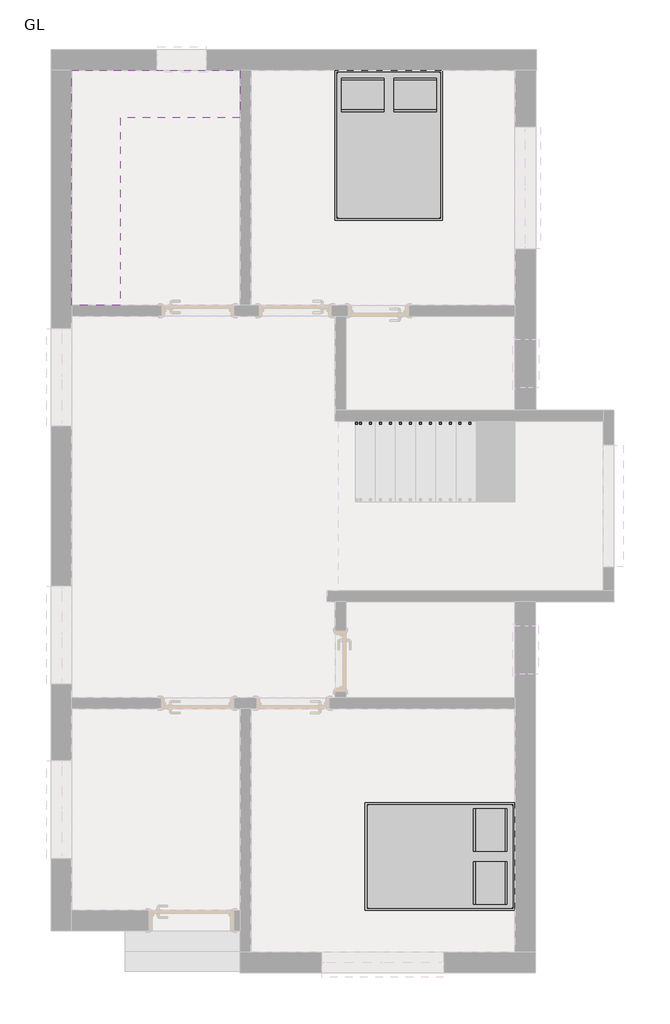
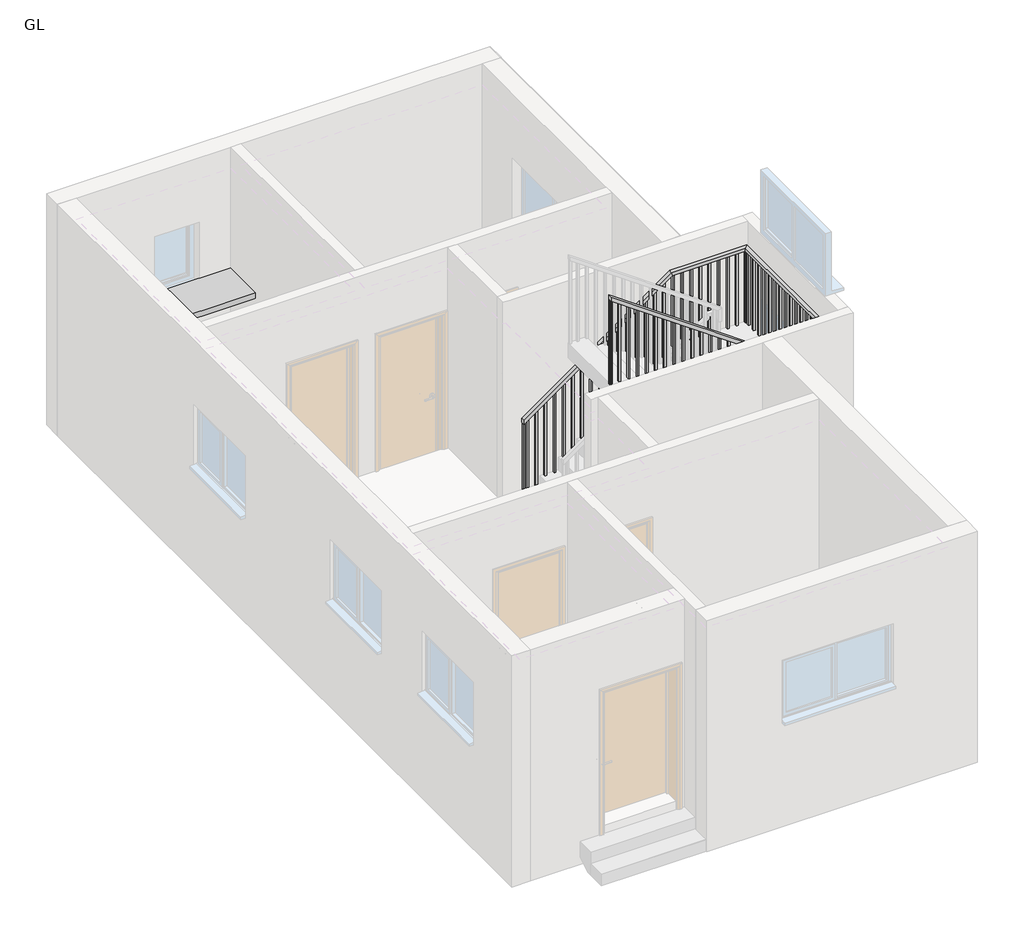
# One storey, part 3 of 3: 2 furniture elements, 1 proxy, 1 railing.
"""IFC4 building model written with IfcOpenShell, lengths in millimetres."""

from ifc_helpers import new_model, si_unit, frame, origin, place, context, project, spatial, polyline, outline, extrude, faceted_brep, transform, mapped, element, save
from components import generic_models_1_generic_models_1_1574f5a2, furniture_bed_1_1346x1880x355mm_double_93dec6ea

model = new_model("IFC4")

# Units and contexts
model_context = context("Model", 3, world=origin())
ifc_project = project(units=[si_unit("LENGTHUNIT", "METRE", prefix="MILLI")], contexts=[model_context])

# Site, building, storey
site = spatial("IfcSite", under=ifc_project)
building = spatial("IfcBuilding", under=site)
storey = spatial("IfcBuildingStorey", under=building, Name="GL", Elevation=0.0)

# Proxy
placement = place(None, origin())
generic_models_1_generic_models_1_shape = generic_models_1_generic_models_1_1574f5a2(model_context)
element("IfcBuildingElementProxy", 1, Name="Generic Models 1 : Generic Models 1", ObjectType="Generic Models 1 : Generic Models 1", at=placement, inside=storey, context=model_context, shape_type="MappedRepresentation", body=[
    mapped(generic_models_1_generic_models_1_shape, transform((0.0, 0.0, 0.0), x_axis=(1.0, 0.0, 0.0), y_axis=(0.0, 1.0, 0.0), z_axis=(0.0, 0.0, 1.0))),
])

# Furniture
furniture_bed_1_1346x1880x355mm_double_shape = furniture_bed_1_1346x1880x355mm_double_93dec6ea(model_context)
element("IfcFurniture", 2, ObjectType="Furniture_Bed_1 : 1346x1880x355mm-Double", at=placement, inside=storey, context=model_context, shape_type="MappedRepresentation", body=[
    mapped(furniture_bed_1_1346x1880x355mm_double_shape, transform((-2224.4098634, 11144.8850079, 149.9616), x_axis=(1.0, 0.0, 0.0), y_axis=(0.0, 1.0, 0.0), z_axis=(0.0, 0.0, 1.0))),
])
element("IfcFurniture", 3, ObjectType="Furniture_Bed_1 : 1346x1880x355mm-Double", at=placement, inside=storey, context=model_context, shape_type="MappedRepresentation", body=[
    mapped(furniture_bed_1_1346x1880x355mm_double_shape, transform((-1007.0378962, 2325.7228167, 149.9616), x_axis=(0.0, -1.0, 0.0), y_axis=(1.0, 0.0, 0.0), z_axis=(0.0, 0.0, 1.0))),
])

# Railing
element("IfcRailing", 4, ObjectType="1100mm", at=placement, inside=storey, context=model_context, shape_type="SolidModel", body=[
    faceted_brep([(-2302.0068409, 7445.8287671, 1279.2941176), (-2302.0068409, 7445.8287671, 1218.028329), (-2302.0068409, 7395.8287671, 1218.028329), (-2302.0068409, 7395.8287671, 1279.2941176), (-276.3568409, 7445.8287671, 2713.6470588), (-260.4468483, 7445.8287671, 2663.6470588), (-260.4468483, 7395.8287671, 2663.6470588), (-276.3568409, 7395.8287671, 2713.6470588), (787.6478774, 7445.8287671, 2713.6470588), (787.6478774, 7445.8287671, 2663.6470588), (737.6478774, 7395.8287671, 2663.6470588), (737.6478774, 7395.8287671, 2713.6470588), (787.6478774, 5318.2803577, 2713.6470588), (787.6478774, 5318.2803577, 2663.6470588), (737.6478774, 5368.2803577, 2663.6470588), (737.6478774, 5368.2803577, 2713.6470588), (-23.1505909, 5318.2803577, 2713.6470588), (-39.0605835, 5318.2803577, 2663.6470588), (-39.0605835, 5368.2803577, 2663.6470588), (-23.1505909, 5368.2803577, 2713.6470588), (-2302.0068409, 5318.2803577, 4327.2941176), (-2302.0068409, 5368.2803577, 4327.2941176), (-2302.0068409, 5368.2803577, 4266.028329), (-2302.0068409, 5318.2803577, 4266.028329)], [[[0, 1, 2, 3]], [[1, 0, 4, 5]], [[2, 1, 5, 6]], [[3, 2, 6, 7]], [[0, 3, 7, 4]], [[5, 4, 8, 9]], [[6, 5, 9, 10]], [[7, 6, 10, 11]], [[4, 7, 11, 8]], [[9, 8, 12, 13]], [[10, 9, 13, 14]], [[11, 10, 14, 15]], [[8, 11, 15, 12]], [[13, 12, 16, 17]], [[14, 13, 17, 18]], [[15, 14, 18, 19]], [[12, 15, 19, 16]], [[20, 21, 22, 23]], [[17, 16, 20, 23]], [[18, 17, 23, 22]], [[19, 18, 22, 21]], [[16, 19, 21, 20]]]),
    extrude(outline(polyline([(4255.6513941, -2287.3521226), (4273.3537729, -2312.3521226), (3048.0, -2312.3521226), (3048.0, -2287.3521226), (4255.6513941, -2287.3521226)])), frame((0.0, 5330.7803577, 0.0), z_axis=(0.0, 1.0, 0.0), x_axis=(0.0, 0.0, 1.0)), (0.0, 0.0, 1.0), 25.0),
    extrude(outline(polyline([(4167.1395003, -2162.3521226), (4184.8418791, -2187.3521226), (3048.0, -2187.3521226), (3048.0, -2162.3521226), (4167.1395003, -2162.3521226)])), frame((0.0, 5330.7803577, 0.0), z_axis=(0.0, 1.0, 0.0), x_axis=(0.0, 0.0, 1.0)), (0.0, 0.0, 1.0), 25.0),
    extrude(outline(polyline([(4078.6276065, -2037.3521226), (4096.3299853, -2062.3521226), (2868.7058824, -2062.3521226), (2868.7058824, -2037.3521226), (4078.6276065, -2037.3521226)])), frame((0.0, 5330.7803577, 0.0), z_axis=(0.0, 1.0, 0.0), x_axis=(0.0, 0.0, 1.0)), (0.0, 0.0, 1.0), 25.0),
    extrude(outline(polyline([(3990.1157127, -1912.3521226), (4007.8180915, -1937.3521226), (2868.7058824, -1937.3521226), (2868.7058824, -1912.3521226), (3990.1157127, -1912.3521226)])), frame((0.0, 5330.7803577, 0.0), z_axis=(0.0, 1.0, 0.0), x_axis=(0.0, 0.0, 1.0)), (0.0, 0.0, 1.0), 25.0),
    extrude(outline(polyline([(3901.603819, -1787.3521226), (3919.3061977, -1812.3521226), (2689.4117647, -1812.3521226), (2689.4117647, -1787.3521226), (3901.603819, -1787.3521226)])), frame((0.0, 5330.7803577, 0.0), z_axis=(0.0, 1.0, 0.0), x_axis=(0.0, 0.0, 1.0)), (0.0, 0.0, 1.0), 25.0),
    extrude(outline(polyline([(3813.0919252, -1662.3521226), (3830.7943039, -1687.3521226), (2689.4117647, -1687.3521226), (2689.4117647, -1662.3521226), (3813.0919252, -1662.3521226)])), frame((0.0, 5330.7803577, 0.0), z_axis=(0.0, 1.0, 0.0), x_axis=(0.0, 0.0, 1.0)), (0.0, 0.0, 1.0), 25.0),
    extrude(outline(polyline([(3724.5800314, -1537.3521226), (3742.2824101, -1562.3521226), (2689.4117647, -1562.3521226), (2689.4117647, -1537.3521226), (3724.5800314, -1537.3521226)])), frame((0.0, 5330.7803577, 0.0), z_axis=(0.0, 1.0, 0.0), x_axis=(0.0, 0.0, 1.0)), (0.0, 0.0, 1.0), 25.0),
    extrude(outline(polyline([(3636.0681376, -1412.3521226), (3653.7705164, -1437.3521226), (2510.1176471, -1437.3521226), (2510.1176471, -1412.3521226), (3636.0681376, -1412.3521226)])), frame((0.0, 5330.7803577, 0.0), z_axis=(0.0, 1.0, 0.0), x_axis=(0.0, 0.0, 1.0)), (0.0, 0.0, 1.0), 25.0),
    extrude(outline(polyline([(3547.5562438, -1287.3521226), (3565.2586226, -1312.3521226), (2510.1176471, -1312.3521226), (2510.1176471, -1287.3521226), (3547.5562438, -1287.3521226)])), frame((0.0, 5330.7803577, 0.0), z_axis=(0.0, 1.0, 0.0), x_axis=(0.0, 0.0, 1.0)), (0.0, 0.0, 1.0), 25.0),
    extrude(outline(polyline([(3459.04435, -1162.3521226), (3476.7467288, -1187.3521226), (2330.8235294, -1187.3521226), (2330.8235294, -1162.3521226), (3459.04435, -1162.3521226)])), frame((0.0, 5330.7803577, 0.0), z_axis=(0.0, 1.0, 0.0), x_axis=(0.0, 0.0, 1.0)), (0.0, 0.0, 1.0), 25.0),
    extrude(outline(polyline([(3370.5324562, -1037.3521226), (3388.234835, -1062.3521226), (2330.8235294, -1062.3521226), (2330.8235294, -1037.3521226), (3370.5324562, -1037.3521226)])), frame((0.0, 5330.7803577, 0.0), z_axis=(0.0, 1.0, 0.0), x_axis=(0.0, 0.0, 1.0)), (0.0, 0.0, 1.0), 25.0),
    extrude(outline(polyline([(3282.0205625, -912.3521226), (3299.7229412, -937.3521226), (2151.5294118, -937.3521226), (2151.5294118, -912.3521226), (3282.0205625, -912.3521226)])), frame((0.0, 5330.7803577, 0.0), z_axis=(0.0, 1.0, 0.0), x_axis=(0.0, 0.0, 1.0)), (0.0, 0.0, 1.0), 25.0),
    extrude(outline(polyline([(3193.5086687, -787.3521226), (3211.2110474, -812.3521226), (2151.5294118, -812.3521226), (2151.5294118, -787.3521226), (3193.5086687, -787.3521226)])), frame((0.0, 5330.7803577, 0.0), z_axis=(0.0, 1.0, 0.0), x_axis=(0.0, 0.0, 1.0)), (0.0, 0.0, 1.0), 25.0),
    extrude(outline(polyline([(3104.9967749, -662.3521226), (3122.6991536, -687.3521226), (1972.2352941, -687.3521226), (1972.2352941, -662.3521226), (3104.9967749, -662.3521226)])), frame((0.0, 5330.7803577, 0.0), z_axis=(0.0, 1.0, 0.0), x_axis=(0.0, 0.0, 1.0)), (0.0, 0.0, 1.0), 25.0),
    extrude(outline(polyline([(3016.4848811, -537.3521226), (3034.1872599, -562.3521226), (1972.2352941, -562.3521226), (1972.2352941, -537.3521226), (3016.4848811, -537.3521226)])), frame((0.0, 5330.7803577, 0.0), z_axis=(0.0, 1.0, 0.0), x_axis=(0.0, 0.0, 1.0)), (0.0, 0.0, 1.0), 25.0),
    extrude(outline(polyline([(2927.9729873, -412.3521226), (2945.6753661, -437.3521226), (1792.9411765, -437.3521226), (1792.9411765, -412.3521226), (2927.9729873, -412.3521226)])), frame((0.0, 5330.7803577, 0.0), z_axis=(0.0, 1.0, 0.0), x_axis=(0.0, 0.0, 1.0)), (0.0, 0.0, 1.0), 25.0),
    extrude(outline(polyline([(2839.4610935, -287.3521226), (2857.1634723, -312.3521226), (1792.9411765, -312.3521226), (1792.9411765, -287.3521226), (2839.4610935, -287.3521226)])), frame((0.0, 5330.7803577, 0.0), z_axis=(0.0, 1.0, 0.0), x_axis=(0.0, 0.0, 1.0)), (0.0, 0.0, 1.0), 25.0),
    extrude(outline(polyline([(2750.9491997, -162.3521226), (2768.6515785, -187.3521226), (1613.6470588, -187.3521226), (1613.6470588, -162.3521226), (2750.9491997, -162.3521226)])), frame((0.0, 5330.7803577, 0.0), z_axis=(0.0, 1.0, 0.0), x_axis=(0.0, 0.0, 1.0)), (0.0, 0.0, 1.0), 25.0),
    extrude(outline(polyline([(2662.437306, -37.3521226), (2680.1396847, -62.3521226), (1613.6470588, -62.3521226), (1613.6470588, -37.3521226), (2662.437306, -37.3521226)])), frame((0.0, 5330.7803577, 0.0), z_axis=(0.0, 1.0, 0.0), x_axis=(0.0, 0.0, 1.0)), (0.0, 0.0, 1.0), 25.0),
    extrude(outline(polyline([(87.6478774, 5330.7803577), (62.6478774, 5330.7803577), (62.6478774, 5355.7803577), (87.6478774, 5355.7803577), (87.6478774, 5330.7803577)])), frame((0.0, 0.0, 1613.6470588), z_axis=(0.0, 0.0, 1.0), x_axis=(1.0, 0.0, 0.0)), (0.0, 0.0, 1.0), 1050.0),
    extrude(outline(polyline([(212.6478774, 5330.7803577), (187.6478774, 5330.7803577), (187.6478774, 5355.7803577), (212.6478774, 5355.7803577), (212.6478774, 5330.7803577)])), frame((0.0, 0.0, 1613.6470588), z_axis=(0.0, 0.0, 1.0), x_axis=(1.0, 0.0, 0.0)), (0.0, 0.0, 1.0), 1050.0),
    extrude(outline(polyline([(337.6478774, 5330.7803577), (312.6478774, 5330.7803577), (312.6478774, 5355.7803577), (337.6478774, 5355.7803577), (337.6478774, 5330.7803577)])), frame((0.0, 0.0, 1613.6470588), z_axis=(0.0, 0.0, 1.0), x_axis=(1.0, 0.0, 0.0)), (0.0, 0.0, 1.0), 1050.0),
    extrude(outline(polyline([(462.6478774, 5330.7803577), (437.6478774, 5330.7803577), (437.6478774, 5355.7803577), (462.6478774, 5355.7803577), (462.6478774, 5330.7803577)])), frame((0.0, 0.0, 1613.6470588), z_axis=(0.0, 0.0, 1.0), x_axis=(1.0, 0.0, 0.0)), (0.0, 0.0, 1.0), 1050.0),
    extrude(outline(polyline([(587.6478774, 5330.7803577), (562.6478774, 5330.7803577), (562.6478774, 5355.7803577), (587.6478774, 5355.7803577), (587.6478774, 5330.7803577)])), frame((0.0, 0.0, 1613.6470588), z_axis=(0.0, 0.0, 1.0), x_axis=(1.0, 0.0, 0.0)), (0.0, 0.0, 1.0), 1050.0),
    extrude(outline(polyline([(712.6478774, 5330.7803577), (687.6478774, 5330.7803577), (687.6478774, 5355.7803577), (712.6478774, 5355.7803577), (712.6478774, 5330.7803577)])), frame((0.0, 0.0, 1613.6470588), z_axis=(0.0, 0.0, 1.0), x_axis=(1.0, 0.0, 0.0)), (0.0, 0.0, 1.0), 1050.0),
    extrude(outline(polyline([(775.1478774, 5370.8287671), (775.1478774, 5345.8287671), (750.1478774, 5345.8287671), (750.1478774, 5370.8287671), (775.1478774, 5370.8287671)])), frame((0.0, 0.0, 1613.6470588), z_axis=(0.0, 0.0, 1.0), x_axis=(1.0, 0.0, 0.0)), (0.0, 0.0, 1.0), 1050.0),
    extrude(outline(polyline([(775.1478774, 5495.8287671), (775.1478774, 5470.8287671), (750.1478774, 5470.8287671), (750.1478774, 5495.8287671), (775.1478774, 5495.8287671)])), frame((0.0, 0.0, 1613.6470588), z_axis=(0.0, 0.0, 1.0), x_axis=(1.0, 0.0, 0.0)), (0.0, 0.0, 1.0), 1050.0),
    extrude(outline(polyline([(775.1478774, 5620.8287671), (775.1478774, 5595.8287671), (750.1478774, 5595.8287671), (750.1478774, 5620.8287671), (775.1478774, 5620.8287671)])), frame((0.0, 0.0, 1613.6470588), z_axis=(0.0, 0.0, 1.0), x_axis=(1.0, 0.0, 0.0)), (0.0, 0.0, 1.0), 1050.0),
    extrude(outline(polyline([(775.1478774, 5745.8287671), (775.1478774, 5720.8287671), (750.1478774, 5720.8287671), (750.1478774, 5745.8287671), (775.1478774, 5745.8287671)])), frame((0.0, 0.0, 1613.6470588), z_axis=(0.0, 0.0, 1.0), x_axis=(1.0, 0.0, 0.0)), (0.0, 0.0, 1.0), 1050.0),
    extrude(outline(polyline([(775.1478774, 5870.8287671), (775.1478774, 5845.8287671), (750.1478774, 5845.8287671), (750.1478774, 5870.8287671), (775.1478774, 5870.8287671)])), frame((0.0, 0.0, 1613.6470588), z_axis=(0.0, 0.0, 1.0), x_axis=(1.0, 0.0, 0.0)), (0.0, 0.0, 1.0), 1050.0),
    extrude(outline(polyline([(775.1478774, 5995.8287671), (775.1478774, 5970.8287671), (750.1478774, 5970.8287671), (750.1478774, 5995.8287671), (775.1478774, 5995.8287671)])), frame((0.0, 0.0, 1613.6470588), z_axis=(0.0, 0.0, 1.0), x_axis=(1.0, 0.0, 0.0)), (0.0, 0.0, 1.0), 1050.0),
    extrude(outline(polyline([(775.1478774, 6120.8287671), (775.1478774, 6095.8287671), (750.1478774, 6095.8287671), (750.1478774, 6120.8287671), (775.1478774, 6120.8287671)])), frame((0.0, 0.0, 1613.6470588), z_axis=(0.0, 0.0, 1.0), x_axis=(1.0, 0.0, 0.0)), (0.0, 0.0, 1.0), 1050.0),
    extrude(outline(polyline([(775.1478774, 6245.8287671), (775.1478774, 6220.8287671), (750.1478774, 6220.8287671), (750.1478774, 6245.8287671), (775.1478774, 6245.8287671)])), frame((0.0, 0.0, 1613.6470588), z_axis=(0.0, 0.0, 1.0), x_axis=(1.0, 0.0, 0.0)), (0.0, 0.0, 1.0), 1050.0),
    extrude(outline(polyline([(775.1478774, 6370.8287671), (775.1478774, 6345.8287671), (750.1478774, 6345.8287671), (750.1478774, 6370.8287671), (775.1478774, 6370.8287671)])), frame((0.0, 0.0, 1613.6470588), z_axis=(0.0, 0.0, 1.0), x_axis=(1.0, 0.0, 0.0)), (0.0, 0.0, 1.0), 1050.0),
    extrude(outline(polyline([(775.1478774, 6495.8287671), (775.1478774, 6470.8287671), (750.1478774, 6470.8287671), (750.1478774, 6495.8287671), (775.1478774, 6495.8287671)])), frame((0.0, 0.0, 1613.6470588), z_axis=(0.0, 0.0, 1.0), x_axis=(1.0, 0.0, 0.0)), (0.0, 0.0, 1.0), 1050.0),
    extrude(outline(polyline([(775.1478774, 6620.8287671), (775.1478774, 6595.8287671), (750.1478774, 6595.8287671), (750.1478774, 6620.8287671), (775.1478774, 6620.8287671)])), frame((0.0, 0.0, 1613.6470588), z_axis=(0.0, 0.0, 1.0), x_axis=(1.0, 0.0, 0.0)), (0.0, 0.0, 1.0), 1050.0),
    extrude(outline(polyline([(775.1478774, 6745.8287671), (775.1478774, 6720.8287671), (750.1478774, 6720.8287671), (750.1478774, 6745.8287671), (775.1478774, 6745.8287671)])), frame((0.0, 0.0, 1613.6470588), z_axis=(0.0, 0.0, 1.0), x_axis=(1.0, 0.0, 0.0)), (0.0, 0.0, 1.0), 1050.0),
    extrude(outline(polyline([(775.1478774, 6870.8287671), (775.1478774, 6845.8287671), (750.1478774, 6845.8287671), (750.1478774, 6870.8287671), (775.1478774, 6870.8287671)])), frame((0.0, 0.0, 1613.6470588), z_axis=(0.0, 0.0, 1.0), x_axis=(1.0, 0.0, 0.0)), (0.0, 0.0, 1.0), 1050.0),
    extrude(outline(polyline([(775.1478774, 6995.8287671), (775.1478774, 6970.8287671), (750.1478774, 6970.8287671), (750.1478774, 6995.8287671), (775.1478774, 6995.8287671)])), frame((0.0, 0.0, 1613.6470588), z_axis=(0.0, 0.0, 1.0), x_axis=(1.0, 0.0, 0.0)), (0.0, 0.0, 1.0), 1050.0),
    extrude(outline(polyline([(775.1478774, 7120.8287671), (775.1478774, 7095.8287671), (750.1478774, 7095.8287671), (750.1478774, 7120.8287671), (775.1478774, 7120.8287671)])), frame((0.0, 0.0, 1613.6470588), z_axis=(0.0, 0.0, 1.0), x_axis=(1.0, 0.0, 0.0)), (0.0, 0.0, 1.0), 1050.0),
    extrude(outline(polyline([(775.1478774, 7245.8287671), (775.1478774, 7220.8287671), (750.1478774, 7220.8287671), (750.1478774, 7245.8287671), (775.1478774, 7245.8287671)])), frame((0.0, 0.0, 1613.6470588), z_axis=(0.0, 0.0, 1.0), x_axis=(1.0, 0.0, 0.0)), (0.0, 0.0, 1.0), 1050.0),
    extrude(outline(polyline([(775.1478774, 7370.8287671), (775.1478774, 7345.8287671), (750.1478774, 7345.8287671), (750.1478774, 7370.8287671), (775.1478774, 7370.8287671)])), frame((0.0, 0.0, 1613.6470588), z_axis=(0.0, 0.0, 1.0), x_axis=(1.0, 0.0, 0.0)), (0.0, 0.0, 1.0), 1050.0),
    extrude(outline(polyline([(747.9931591, 7433.3287671), (772.9931591, 7433.3287671), (772.9931591, 7408.3287671), (747.9931591, 7408.3287671), (747.9931591, 7433.3287671)])), frame((0.0, 0.0, 1613.6470588), z_axis=(0.0, 0.0, 1.0), x_axis=(1.0, 0.0, 0.0)), (0.0, 0.0, 1.0), 1050.0),
    extrude(outline(polyline([(622.9931591, 7433.3287671), (647.9931591, 7433.3287671), (647.9931591, 7408.3287671), (622.9931591, 7408.3287671), (622.9931591, 7433.3287671)])), frame((0.0, 0.0, 1613.6470588), z_axis=(0.0, 0.0, 1.0), x_axis=(1.0, 0.0, 0.0)), (0.0, 0.0, 1.0), 1050.0),
    extrude(outline(polyline([(497.9931591, 7433.3287671), (522.9931591, 7433.3287671), (522.9931591, 7408.3287671), (497.9931591, 7408.3287671), (497.9931591, 7433.3287671)])), frame((0.0, 0.0, 1613.6470588), z_axis=(0.0, 0.0, 1.0), x_axis=(1.0, 0.0, 0.0)), (0.0, 0.0, 1.0), 1050.0),
    extrude(outline(polyline([(372.9931591, 7433.3287671), (397.9931591, 7433.3287671), (397.9931591, 7408.3287671), (372.9931591, 7408.3287671), (372.9931591, 7433.3287671)])), frame((0.0, 0.0, 1613.6470588), z_axis=(0.0, 0.0, 1.0), x_axis=(1.0, 0.0, 0.0)), (0.0, 0.0, 1.0), 1050.0),
    extrude(outline(polyline([(247.9931591, 7433.3287671), (272.9931591, 7433.3287671), (272.9931591, 7408.3287671), (247.9931591, 7408.3287671), (247.9931591, 7433.3287671)])), frame((0.0, 0.0, 1613.6470588), z_axis=(0.0, 0.0, 1.0), x_axis=(1.0, 0.0, 0.0)), (0.0, 0.0, 1.0), 1050.0),
    extrude(outline(polyline([(122.9931591, 7433.3287671), (147.9931591, 7433.3287671), (147.9931591, 7408.3287671), (122.9931591, 7408.3287671), (122.9931591, 7433.3287671)])), frame((0.0, 0.0, 1613.6470588), z_axis=(0.0, 0.0, 1.0), x_axis=(1.0, 0.0, 0.0)), (0.0, 0.0, 1.0), 1050.0),
    extrude(outline(polyline([(-2.0068409, 7433.3287671), (22.9931591, 7433.3287671), (22.9931591, 7408.3287671), (-2.0068409, 7408.3287671), (-2.0068409, 7433.3287671)])), frame((0.0, 0.0, 1613.6470588), z_axis=(0.0, 0.0, 1.0), x_axis=(1.0, 0.0, 0.0)), (0.0, 0.0, 1.0), 1050.0),
    extrude(outline(polyline([(-127.0068409, 7433.3287671), (-102.0068409, 7433.3287671), (-102.0068409, 7408.3287671), (-127.0068409, 7408.3287671), (-127.0068409, 7433.3287671)])), frame((0.0, 0.0, 1613.6470588), z_axis=(0.0, 0.0, 1.0), x_axis=(1.0, 0.0, 0.0)), (0.0, 0.0, 1.0), 1050.0),
    extrude(outline(polyline([(-252.0068409, 7433.3287671), (-227.0068409, 7433.3287671), (-227.0068409, 7408.3287671), (-252.0068409, 7408.3287671), (-252.0068409, 7433.3287671)])), frame((0.0, 0.0, 1613.6470588), z_axis=(0.0, 0.0, 1.0), x_axis=(1.0, 0.0, 0.0)), (0.0, 0.0, 1.0), 1050.0),
    extrude(outline(polyline([(1434.3529412, -377.0068409), (1434.3529412, -352.0068409), (2598.8138721, -352.0068409), (2581.1114933, -377.0068409), (1434.3529412, -377.0068409)])), frame((0.0, 7408.3287671, 0.0), z_axis=(0.0, 1.0, 0.0), x_axis=(0.0, 0.0, 1.0)), (0.0, 0.0, 1.0), 25.0),
    extrude(outline(polyline([(1434.3529412, -502.0068409), (1434.3529412, -477.0068409), (2510.3019783, -477.0068409), (2492.5995995, -502.0068409), (1434.3529412, -502.0068409)])), frame((0.0, 7408.3287671, 0.0), z_axis=(0.0, 1.0, 0.0), x_axis=(0.0, 0.0, 1.0)), (0.0, 0.0, 1.0), 25.0),
    extrude(outline(polyline([(1255.0588235, -627.0068409), (1255.0588235, -602.0068409), (2421.7900845, -602.0068409), (2404.0877058, -627.0068409), (1255.0588235, -627.0068409)])), frame((0.0, 7408.3287671, 0.0), z_axis=(0.0, 1.0, 0.0), x_axis=(0.0, 0.0, 1.0)), (0.0, 0.0, 1.0), 25.0),
    extrude(outline(polyline([(1255.0588235, -752.0068409), (1255.0588235, -727.0068409), (2333.2781907, -727.0068409), (2315.575812, -752.0068409), (1255.0588235, -752.0068409)])), frame((0.0, 7408.3287671, 0.0), z_axis=(0.0, 1.0, 0.0), x_axis=(0.0, 0.0, 1.0)), (0.0, 0.0, 1.0), 25.0),
    extrude(outline(polyline([(1075.7647059, -877.0068409), (1075.7647059, -852.0068409), (2244.7662969, -852.0068409), (2227.0639182, -877.0068409), (1075.7647059, -877.0068409)])), frame((0.0, 7408.3287671, 0.0), z_axis=(0.0, 1.0, 0.0), x_axis=(0.0, 0.0, 1.0)), (0.0, 0.0, 1.0), 25.0),
    extrude(outline(polyline([(1075.7647059, -1002.0068409), (1075.7647059, -977.0068409), (2156.2544032, -977.0068409), (2138.5520244, -1002.0068409), (1075.7647059, -1002.0068409)])), frame((0.0, 7408.3287671, 0.0), z_axis=(0.0, 1.0, 0.0), x_axis=(0.0, 0.0, 1.0)), (0.0, 0.0, 1.0), 25.0),
    extrude(outline(polyline([(896.4705882, -1127.0068409), (896.4705882, -1102.0068409), (2067.7425094, -1102.0068409), (2050.0401306, -1127.0068409), (896.4705882, -1127.0068409)])), frame((0.0, 7408.3287671, 0.0), z_axis=(0.0, 1.0, 0.0), x_axis=(0.0, 0.0, 1.0)), (0.0, 0.0, 1.0), 25.0),
    extrude(outline(polyline([(896.4705882, -1252.0068409), (896.4705882, -1227.0068409), (1979.2306156, -1227.0068409), (1961.5282368, -1252.0068409), (896.4705882, -1252.0068409)])), frame((0.0, 7408.3287671, 0.0), z_axis=(0.0, 1.0, 0.0), x_axis=(0.0, 0.0, 1.0)), (0.0, 0.0, 1.0), 25.0),
    extrude(outline(polyline([(717.1764706, -1377.0068409), (717.1764706, -1352.0068409), (1890.7187218, -1352.0068409), (1873.016343, -1377.0068409), (717.1764706, -1377.0068409)])), frame((0.0, 7408.3287671, 0.0), z_axis=(0.0, 1.0, 0.0), x_axis=(0.0, 0.0, 1.0)), (0.0, 0.0, 1.0), 25.0),
    extrude(outline(polyline([(717.1764706, -1502.0068409), (717.1764706, -1477.0068409), (1802.206828, -1477.0068409), (1784.5044493, -1502.0068409), (717.1764706, -1502.0068409)])), frame((0.0, 7408.3287671, 0.0), z_axis=(0.0, 1.0, 0.0), x_axis=(0.0, 0.0, 1.0)), (0.0, 0.0, 1.0), 25.0),
    extrude(outline(polyline([(537.8823529, -1627.0068409), (537.8823529, -1602.0068409), (1713.6949342, -1602.0068409), (1695.9925555, -1627.0068409), (537.8823529, -1627.0068409)])), frame((0.0, 7408.3287671, 0.0), z_axis=(0.0, 1.0, 0.0), x_axis=(0.0, 0.0, 1.0)), (0.0, 0.0, 1.0), 25.0),
    extrude(outline(polyline([(537.8823529, -1752.0068409), (537.8823529, -1727.0068409), (1625.1830404, -1727.0068409), (1607.4806617, -1752.0068409), (537.8823529, -1752.0068409)])), frame((0.0, 7408.3287671, 0.0), z_axis=(0.0, 1.0, 0.0), x_axis=(0.0, 0.0, 1.0)), (0.0, 0.0, 1.0), 25.0),
    extrude(outline(polyline([(358.5882353, -1877.0068409), (358.5882353, -1852.0068409), (1536.6711467, -1852.0068409), (1518.9687679, -1877.0068409), (358.5882353, -1877.0068409)])), frame((0.0, 7408.3287671, 0.0), z_axis=(0.0, 1.0, 0.0), x_axis=(0.0, 0.0, 1.0)), (0.0, 0.0, 1.0), 25.0),
    extrude(outline(polyline([(358.5882353, -2002.0068409), (358.5882353, -1977.0068409), (1448.1592529, -1977.0068409), (1430.4568741, -2002.0068409), (358.5882353, -2002.0068409)])), frame((0.0, 7408.3287671, 0.0), z_axis=(0.0, 1.0, 0.0), x_axis=(0.0, 0.0, 1.0)), (0.0, 0.0, 1.0), 25.0),
    extrude(outline(polyline([(179.2941176, -2127.0068409), (179.2941176, -2102.0068409), (1359.6473591, -2102.0068409), (1341.9449803, -2127.0068409), (179.2941176, -2127.0068409)])), frame((0.0, 7408.3287671, 0.0), z_axis=(0.0, 1.0, 0.0), x_axis=(0.0, 0.0, 1.0)), (0.0, 0.0, 1.0), 25.0),
    extrude(outline(polyline([(179.2941176, -2252.0068409), (179.2941176, -2227.0068409), (1271.1354653, -2227.0068409), (1253.4330865, -2252.0068409), (179.2941176, -2252.0068409)])), frame((0.0, 7408.3287671, 0.0), z_axis=(0.0, 1.0, 0.0), x_axis=(0.0, 0.0, 1.0)), (0.0, 0.0, 1.0), 25.0),
    extrude(outline(polyline([(775.1478774, 5355.7803577), (775.1478774, 5330.7803577), (750.1478774, 5330.7803577), (750.1478774, 5355.7803577), (775.1478774, 5355.7803577)])), frame((0.0, 0.0, 1613.6470588), z_axis=(0.0, 0.0, 1.0), x_axis=(1.0, 0.0, 0.0)), (0.0, 0.0, 1.0), 1050.0),
    extrude(outline(polyline([(750.1478774, 7433.3287671), (775.1478774, 7433.3287671), (775.1478774, 7408.3287671), (750.1478774, 7408.3287671), (750.1478774, 7433.3287671)])), frame((0.0, 0.0, 1613.6470588), z_axis=(0.0, 0.0, 1.0), x_axis=(1.0, 0.0, 0.0)), (0.0, 0.0, 1.0), 1050.0),
    extrude(outline(polyline([(4248.3259503, -2277.0068409), (4266.028329, -2302.0068409), (3048.0, -2302.0068409), (3048.0, -2277.0068409), (4248.3259503, -2277.0068409)])), frame((0.0, 5330.7803577, 0.0), z_axis=(0.0, 1.0, 0.0), x_axis=(0.0, 0.0, 1.0)), (0.0, 0.0, 1.0), 25.0),
    extrude(outline(polyline([(179.2941176, -2302.0068409), (179.2941176, -2277.0068409), (1235.7307078, -2277.0068409), (1218.028329, -2302.0068409), (179.2941176, -2302.0068409)])), frame((0.0, 7408.3287671, 0.0), z_axis=(0.0, 1.0, 0.0), x_axis=(0.0, 0.0, 1.0)), (0.0, 0.0, 1.0), 25.0),
])

save(model, "model.ifc")

# Revit data of these elements
# Type "Furniture_Bed_1 : 1346x1880x355mm-Double"
#   Keynote = "N"
#   Length = 1880 mm
#   Width = 1346 mm
#   Material Frame = Wood - Birch
#   Material Mattress = Textile - White
#   Default Elevation = 0
# Type "1100mm"
#   built-in parameter 1008612 = 0.019685 (stored number, unit not read)
#   built-in parameter 1008611 = 0.019685 (stored number, unit not read)
#   built-in parameter 1008609 = 0.902231 (stored number, unit not read)
#   built-in parameter 1008604 = 0.19685 (stored number, unit not read)
#   built-in parameter 1008603 = 0.164042 (stored number, unit not read)
#   Railing Height = 1100 mm
#   built-in parameter 1008630 = 2
#   built-in parameter 1008610 = 2
#   built-in parameter 1008608 = 1
#   built-in parameter 1008618 = Baluster_Square : 25mm
# Element 1 (IfcBuildingElementProxy, "Generic Models 1 : Generic Models 1")
#   Phase Created = New Construction
#   Materials on its faces: "Concrete, Precast"
# Elements 2, 3 (IfcFurniture, "Furniture_Bed_1 : 1346x1880x355mm-Double")
#   Phase Created = New Construction
#   Materials on its faces: "Wood - Birch", "Textile - White"
# Element 4 (IfcRailing, "1100mm")
#   Phase Created = New Construction
# Materials
#   "Wood - Birch": class "Wood", colour RGB 224 178 126, transparency 0
#   "Textile - White": class "Fabric", colour RGB 247 247 239, transparency 0
#   "Concrete, Precast": class "Concrete", colour RGB 192 192 192, transparency 0, Description = "Precast concrete", Cost = 0
